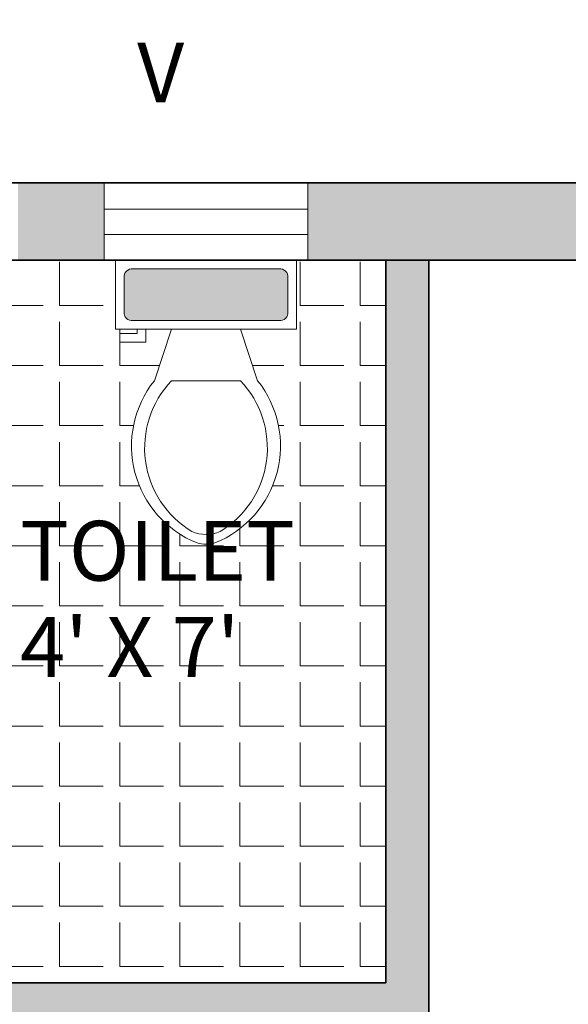
# Model space of a CAD drawing. Units: inches. Extents: x 1858 to 2399, y 1317 to 1943.
# Tile 5 of 8: x 2098 to 2162, y 1742 to 1856. Entities that reach past the tile are written whole.
import ezdxf

# ---------------------------------------------------------------- set-up
doc = ezdxf.new("R2010")
doc.units = ezdxf.units.IN
for name, color, linetype, lineweight in [('A-ANNO-DIMS', 2, 'Continuous', 18), ('A-ANNO-TEXT', 7, 'Continuous', 18), ('A-AREA-IDEN', 7, 'Continuous', 18), ('A-FLOR-FIXT', 9, 'Continuous', 18), ('A-FLOR-FIXT-PATT', 9, 'Continuous', 13), ('A-FLOR-PATT', 8, 'Continuous', 13), ('A-WALL', 7, 'Continuous', 35), ('A-WALL-PATT', 1, 'Continuous', 13), ('window', 4, 'Continuous', 18)]:
    doc.layers.add(name, color=color, linetype=linetype, lineweight=lineweight)
doc.styles.get("Standard").update_dxf_attribs({"font": 'arial.ttf'})
doc.dimstyles.new('ISO-25', dxfattribs={"dimtxt": 12.5, "dimasz": 2.5, "dimexe": 1.25, "dimexo": 0.625, "dimtad": 1, "dimdec": 0, "dimlunit": 4, "dimtxsty": 'Standard', "dimblk": 'ARCHTICK', "dimcen": 2.5, "dimse1": 1, "dimse2": 1, "dimclrd": 3, "dimclrt": 4, "dimadec": 0, "dimazin": 0, "dimtfac": 1, "dimtdec": 0, "dimtmove": 0, "dimatfit": 3, "dimfxl": 1, "dimarcsym": 0})

# ---------------------------------------------------------------- blocks, each defined once
blk = doc.blocks.new('*U4')
for p, q in [((9.5, -6), (9.5, -2)), ((-8, -8.5), (-8, -8)), ((-7, -8), (-7, -9.5)), ((-4, -8), (-6, -14)), ((4, -8), (6, -14)), ((-10, -8.5), (-8, -8.5)), ((-10, -9.5), (-10, -8.5)), ((-7, -9.5), (-10, -9.5)), ((4, -14), (-4, -14))]:
    blk.add_line(p, q)
blk.add_lwpolyline([(10.5, -8), (10.5, 0), (-10.5, 0), (-10.5, -8)], close=True)
for points in [[(8.5, -1), (-8.5, -1)], [(-9.5, -2), (-9.5, -6)], [(-8.5, -7), (8.5, -7)]]:
    blk.add_lwpolyline(points)
for centre, radius, start, end in [((-8.62, -1.88), 0.884, 81.8699, 188.1301), ((8.62, -1.88), 0.884, 351.8699, 98.1301), ((-8.62, -6.12), 0.884, 171.8699, 278.1301), ((8.62, -6.12), 0.884, 261.8699, 8.1301), ((3.52, -21.58), 12.17, 141.4691, 247.9714), ((4.2, -21.82), 11.33, 136.3677, 238.9468), ((-3.52, -21.58), 12.17, 292.0284, 38.5307), ((-4.2, -21.82), 11.33, 301.053, 43.6321), ((0, -27.88), 4, 245.7318, 294.2682), ((0, -29), 4, 254.8605, 285.1395)]:
    blk.add_arc(centre, radius, start, end)
blk = doc.blocks.new('_ArchTick')
at = {"color": 0, "linetype": 'ByBlock', "const_width": 0.15}
blk.add_lwpolyline([(-0.5, -0.5), (0.5, 0.5)], dxfattribs=at)
blk = doc.blocks.new('*D14')
at = {"layer": 'A-ANNO-DIMS', "color": 0, "lineweight": -2, "transparency": 16777216}
blk.add_line((1913.38, 1886.42), (2273.38, 1886.42), dxfattribs=at)
at = {"layer": 'Defpoints', "color": 0, "transparency": 16777216}
for p in [(2273.38, 1886.42), (2273.38, 1827.14), (1913.38, 1826.41)]:
    blk.add_point(p, dxfattribs=at)
at = {"layer": 'A-ANNO-DIMS', "color": 0, "lineweight": -2, "transparency": 16777216, "xscale": 2.5, "yscale": 2.5, "zscale": 2.5, "rotation": 180}
blk.add_blockref('_ArchTick', (1913.38, 1886.42), dxfattribs=at)
at = {"layer": 'A-ANNO-DIMS', "color": 0, "lineweight": -2, "transparency": 16777216, "xscale": 2.5, "yscale": 2.5, "zscale": 2.5}
blk.add_blockref('_ArchTick', (2273.38, 1886.42), dxfattribs=at)
at = {"layer": 'A-ANNO-DIMS', "color": 0, "transparency": 16777216, "insert": (2093.38, 1893.43), "char_height": 12.5, "attachment_point": 5}
blk.add_mtext("30'", dxfattribs=at)
blk = doc.blocks.new('*D33')
at = {"layer": 'A-ANNO-DIMS', "color": 3, "lineweight": -2, "transparency": 16777216}
for p, q in [((1989.86, 1917.54), (2051.43, 1917.54)), ((2051.43, 1917.54), (2117.53, 1917.54))]:
    blk.add_line(p, q, dxfattribs=at)
at = {"layer": 'Defpoints', "color": 0, "transparency": 16777216}
for p in [(2051.43, 1917.54), (1989.86, 1837.34), (2051.43, 1837.34)]:
    blk.add_point(p, dxfattribs=at)
at = {"layer": 'A-ANNO-DIMS', "color": 3, "lineweight": -2, "transparency": 16777216, "xscale": 2.5, "yscale": 2.5, "zscale": 2.5, "rotation": 180}
blk.add_blockref('_ArchTick', (1989.86, 1917.54), dxfattribs=at)
at = {"layer": 'A-ANNO-DIMS', "color": 3, "lineweight": -2, "transparency": 16777216, "xscale": 2.5, "yscale": 2.5, "zscale": 2.5}
blk.add_blockref('_ArchTick', (2051.43, 1917.54), dxfattribs=at)
at = {"layer": 'A-ANNO-DIMS', "color": 4, "transparency": 16777216, "insert": (2085.73, 1924.63), "char_height": 12.5, "attachment_point": 5}
blk.add_mtext('5\'-1 1/2"', dxfattribs=at)
blk = doc.blocks.new('*D34')
at = {"layer": 'A-ANNO-DIMS', "color": 3, "lineweight": -2, "transparency": 16777216}
blk.add_line((2051.43, 1917.54), (2107.67, 1917.54), dxfattribs=at)
at = {"layer": 'Defpoints', "color": 0, "transparency": 16777216}
for p in [(2107.67, 1917.54), (2051.43, 1837.34), (2107.67, 1837.34)]:
    blk.add_point(p, dxfattribs=at)
at = {"layer": 'A-ANNO-DIMS', "color": 3, "lineweight": -2, "transparency": 16777216, "xscale": 2.5, "yscale": 2.5, "zscale": 2.5, "rotation": 180}
blk.add_blockref('_ArchTick', (2051.43, 1917.54), dxfattribs=at)
at = {"layer": 'A-ANNO-DIMS', "color": 3, "lineweight": -2, "transparency": 16777216, "xscale": 2.5, "yscale": 2.5, "zscale": 2.5}
blk.add_blockref('_ArchTick', (2107.67, 1917.54), dxfattribs=at)
at = {"layer": 'A-ANNO-DIMS', "color": 4, "transparency": 16777216, "insert": (2079.55, 1924.55), "char_height": 12.5, "attachment_point": 5}
blk.add_mtext('4\'-8"', dxfattribs=at)
blk = doc.blocks.new('*D35')
at = {"layer": 'A-ANNO-DIMS', "color": 3, "lineweight": -2, "transparency": 16777216}
for p, q in [((2107.67, 1917.54), (2131.33, 1917.54)), ((2131.33, 1917.54), (2205.97, 1917.54))]:
    blk.add_line(p, q, dxfattribs=at)
at = {"layer": 'Defpoints', "color": 0, "transparency": 16777216}
for p in [(2131.33, 1917.54), (2107.67, 1837.34), (2131.33, 1837.34)]:
    blk.add_point(p, dxfattribs=at)
at = {"layer": 'A-ANNO-DIMS', "color": 3, "lineweight": -2, "transparency": 16777216, "xscale": 2.5, "yscale": 2.5, "zscale": 2.5, "rotation": 180}
blk.add_blockref('_ArchTick', (2107.67, 1917.54), dxfattribs=at)
at = {"layer": 'A-ANNO-DIMS', "color": 3, "lineweight": -2, "transparency": 16777216, "xscale": 2.5, "yscale": 2.5, "zscale": 2.5}
blk.add_blockref('_ArchTick', (2131.33, 1917.54), dxfattribs=at)
at = {"layer": 'A-ANNO-DIMS', "color": 4, "transparency": 16777216, "insert": (2169.9, 1924.63), "char_height": 12.5, "attachment_point": 5}
blk.add_mtext('1\'-11 1/2"', dxfattribs=at)
blk = doc.blocks.new('*D36')
at = {"layer": 'A-ANNO-DIMS', "color": 3, "lineweight": -2, "transparency": 16777216}
for p, q in [((2131.33, 1917.54), (2186.7, 1917.54)), ((2186.7, 1917.54), (2253.31, 1917.54))]:
    blk.add_line(p, q, dxfattribs=at)
at = {"layer": 'Defpoints', "color": 0, "transparency": 16777216}
for p in [(2186.7, 1917.54), (2131.33, 1837.34), (2186.7, 1837.34)]:
    blk.add_point(p, dxfattribs=at)
at = {"layer": 'A-ANNO-DIMS', "color": 3, "lineweight": -2, "transparency": 16777216, "xscale": 2.5, "yscale": 2.5, "zscale": 2.5, "rotation": 180}
blk.add_blockref('_ArchTick', (2131.33, 1917.54), dxfattribs=at)
at = {"layer": 'A-ANNO-DIMS', "color": 3, "lineweight": -2, "transparency": 16777216, "xscale": 2.5, "yscale": 2.5, "zscale": 2.5}
blk.add_blockref('_ArchTick', (2186.7, 1917.54), dxfattribs=at)
at = {"layer": 'A-ANNO-DIMS', "color": 4, "transparency": 16777216, "insert": (2221.25, 1924.63), "char_height": 12.5, "attachment_point": 5}
blk.add_mtext('4\'-7 1/2"', dxfattribs=at)
blk = doc.blocks.new('*D50')
at = {"layer": 'A-ANNO-DIMS', "color": 3, "lineweight": -2, "transparency": 16777216}
for p, q in [((2097.46, 1917.54), (2127.41, 1917.54)), ((2127.41, 1917.54), (2164.6, 1917.54))]:
    blk.add_line(p, q, dxfattribs=at)
at = {"layer": 'Defpoints', "color": 0, "transparency": 16777216}
for p in [(2127.41, 1917.54), (2097.46, 1563.34), (2127.41, 1563.34)]:
    blk.add_point(p, dxfattribs=at)
at = {"layer": 'A-ANNO-DIMS', "color": 3, "lineweight": -2, "transparency": 16777216, "xscale": 2.5, "yscale": 2.5, "zscale": 2.5, "rotation": 180}
blk.add_blockref('_ArchTick', (2097.46, 1917.54), dxfattribs=at)
at = {"layer": 'A-ANNO-DIMS', "color": 3, "lineweight": -2, "transparency": 16777216, "xscale": 2.5, "yscale": 2.5, "zscale": 2.5}
blk.add_blockref('_ArchTick', (2127.41, 1917.54), dxfattribs=at)
at = {"layer": 'A-ANNO-DIMS', "color": 4, "transparency": 16777216, "insert": (2147.25, 1924.55), "char_height": 12.5, "attachment_point": 5}
blk.add_mtext('2\'-6"', dxfattribs=at)
blk = doc.blocks.new('*D51')
at = {"layer": 'A-ANNO-DIMS', "color": 3, "lineweight": -2, "transparency": 16777216}
for p, q in [((2127.41, 1917.54), (2171.86, 1917.54)), ((2171.86, 1917.54), (2237.95, 1917.54))]:
    blk.add_line(p, q, dxfattribs=at)
at = {"layer": 'Defpoints', "color": 0, "transparency": 16777216}
for p in [(2171.86, 1917.54), (2127.41, 1563.34), (2171.86, 1563.34)]:
    blk.add_point(p, dxfattribs=at)
at = {"layer": 'A-ANNO-DIMS', "color": 3, "lineweight": -2, "transparency": 16777216, "xscale": 2.5, "yscale": 2.5, "zscale": 2.5, "rotation": 180}
blk.add_blockref('_ArchTick', (2127.41, 1917.54), dxfattribs=at)
at = {"layer": 'A-ANNO-DIMS', "color": 3, "lineweight": -2, "transparency": 16777216, "xscale": 2.5, "yscale": 2.5, "zscale": 2.5}
blk.add_blockref('_ArchTick', (2171.86, 1917.54), dxfattribs=at)
at = {"layer": 'A-ANNO-DIMS', "color": 4, "transparency": 16777216, "insert": (2206.15, 1924.63), "char_height": 12.5, "attachment_point": 5}
blk.add_mtext('3\'-8 1/2"', dxfattribs=at)
blk = doc.blocks.new('*D58')
at = {"layer": 'A-ANNO-DIMS', "color": 3, "lineweight": -2, "transparency": 16777216}
for p, q in [((1884.18, 1730.57), (1884.18, 1767.76)), ((1884.18, 1706.78), (1884.18, 1730.57))]:
    blk.add_line(p, q, dxfattribs=at)
at = {"layer": 'Defpoints', "color": 0, "transparency": 16777216}
for p in [(1884.18, 1730.57), (2145.38, 1730.57), (2145.38, 1706.78)]:
    blk.add_point(p, dxfattribs=at)
at = {"layer": 'A-ANNO-DIMS', "color": 3, "lineweight": -2, "transparency": 16777216, "xscale": 2.5, "yscale": 2.5, "zscale": 2.5}
for p, rotation in [((1884.18, 1730.57), 90), ((1884.18, 1706.78), 270)]:
    blk.add_blockref('_ArchTick', p, dxfattribs=dict(at, rotation=rotation))
at = {"layer": 'A-ANNO-DIMS', "color": 4, "transparency": 16777216, "insert": (1877.17, 1750.41), "char_height": 12.5, "attachment_point": 5, "rotation": 90}
blk.add_mtext('2\'-0"', dxfattribs=at)

msp = doc.modelspace()

# ---------------------------------------------------------------- hatches: boundary and pattern name
at = {"layer": 'A-FLOR-FIXT-PATT'}
h = msp.add_hatch(color=256, dxfattribs=at)
h.dxf.hatch_style = 1
h.set_gradient(color1=(0, 0, 255), color2=(255, 255, 0))
h.paths.add_polyline_path([(2010.03, 1501.34), (2040.03, 1501.34), (2040.03, 1477.34), (2034.03, 1477.34), (2034.03, 1476.34), (2038.03, 1476.34), (2050.44, 1476.34), (2056.5, 1476.34), (2056.5, 1507.28), (1988.35, 1507.28), (1988.35, 1554.34), (1967.38, 1554.34), (1967.38, 1525.7, -0.414214), (1968.88, 1527.2), (1985.88, 1527.2, -0.414214), (1987.38, 1525.7), (1987.38, 1498.7, -0.414214), (1985.88, 1497.2), (1968.88, 1497.2, -0.414214), (1967.38, 1498.7), (1967.38, 1476.34), (2016.03, 1476.34), (2016.03, 1477.34), (2010.03, 1477.34)])
h.paths.add_polyline_path([(2129, 1826.59, 0.414214), (2128, 1827.34), (2110.75, 1827.34, 0.414214), (2110, 1826.34), (2110, 1822.09, 0.414214), (2111, 1821.34), (2128.25, 1821.34, 0.414214), (2129, 1822.34)])
h.paths.add_polyline_path([(2047.65, 1651.34), (2026.65, 1651.34), (2026.65, 1643.34), (2047.65, 1643.34)])
h.paths.add_polyline_path([(2045.65, 1644.34, 0.5), (2046.65, 1645.34), (2046.65, 1649.34, 0.5), (2045.65, 1650.34), (2028.65, 1650.34, 0.5), (2027.65, 1649.34), (2027.65, 1645.34, 0.5), (2028.65, 1644.34)], flags=16)
at = {"layer": 'A-FLOR-PATT'}
h = msp.add_hatch(dxfattribs=at)
h.set_pattern_fill('ANGLE', color=256)
h.set_pattern_definition([(0, (0, 0), (0, 6.985), [5.08, -1.905]), (90, (0, 0), (-6.985, 4e-16), [5.08, -1.905])])
h.paths.add_polyline_path([(2058.38, 1691.34), (2005.38, 1691.34), (2005.38, 1696.34), (1977.99, 1696.34), (1977.99, 1691.34), (1967.38, 1691.34), (1967.38, 1643.34), (2026.65, 1643.34), (2026.65, 1651.34), (2033.15, 1651.34), (2031.15, 1657.34, -0.501323), (2036.1, 1676.2, -0.132891), (2038.19, 1676.2, -0.501317), (2043.15, 1657.34), (2041.15, 1651.34), (2044.15, 1651.34), (2044.15, 1652.84), (2047.15, 1652.84), (2047.15, 1651.34), (2047.65, 1651.34), (2047.65, 1643.34), (2058.38, 1643.34)])
h.paths.add_polyline_path([(2140.38, 1828.34), (2130, 1828.34), (2130, 1820.34), (2123.5, 1820.34), (2125.5, 1814.34, -0.501323), (2120.55, 1795.48, -0.132891), (2118.46, 1795.48, -0.501317), (2113.5, 1814.34), (2115.5, 1820.34), (2112.5, 1820.34), (2112.5, 1818.84), (2109.5, 1818.84), (2109.5, 1820.34), (2109, 1820.34), (2109, 1828.34), (2107.67, 1828.34), (2092.38, 1828.34), (2092.38, 1744.34), (2140.38, 1744.34)])
h.paths.add_polyline_path([(1981.03, 1683.02), (1996.96, 1683.02), (1996.96, 1693.5), (1981.03, 1693.5)], flags=24)
h.paths.add_polyline_path([(1975.79, 1660.59), (2014.55, 1660.59), (2014.55, 1671.04), (1975.79, 1671.04)], flags=24)
h.paths.add_polyline_path([(1975.73, 1671.6), (2013.37, 1671.6), (2013.37, 1682.41), (1975.73, 1682.41)], flags=24)
h.paths.add_polyline_path([(2096.15, 1778.17), (2126.05, 1778.17), (2126.05, 1788.61), (2096.15, 1788.61)], flags=24)
h.paths.add_polyline_path([(2096.09, 1789.17), (2133.73, 1789.17), (2133.73, 1799.98), (2096.09, 1799.98)], flags=24)
at = {"layer": 'A-WALL-PATT'}
h = msp.add_hatch(color=256, dxfattribs=at)
h.dxf.hatch_style = 1
h.paths.add_polyline_path([(1967.38, 1742.58), (1958.38, 1742.58), (1958.38, 1700.89), (1967.38, 1700.89)])
h.paths.add_polyline_path([(1967.38, 1685.05), (1958.38, 1685.05), (1958.38, 1672.42), (1967.38, 1672.42)], flags=17)
h.paths.add_polyline_path([(2092.38, 1643.34), (2087.38, 1643.34), (2063.38, 1643.34), (2063.38, 1691.34), (2087.38, 1691.34), (2092.38, 1691.34), (2092.38, 1696.34), (2087.38, 1696.34), (2005.38, 1696.34), (2005.38, 1691.34), (2058.38, 1691.34), (2058.38, 1643.34), (1967.38, 1643.34), (1967.38, 1652.51), (1958.38, 1652.51), (1958.38, 1625.4), (1967.38, 1625.4), (1967.38, 1638.34), (2087.38, 1638.34), (2087.38, 1617.63), (2092.38, 1617.63)])
h.paths.add_polyline_path([(1967.38, 1591.74), (1958.38, 1591.74), (1958.38, 1571.83), (1967.38, 1571.83)])
h.paths.add_polyline_path([(1967.38, 1554.34), (2002.1, 1554.34), (2002.1, 1559.34), (1967.38, 1559.34), (1958.38, 1559.34), (1958.38, 1536.07), (1967.38, 1536.07)])
h.paths.add_polyline_path([(2087.38, 1559.34), (2042.3, 1559.34), (2042.3, 1554.34), (2087.38, 1554.34)])
h.paths.add_polyline_path([(2092.38, 1583.24), (2087.38, 1583.24), (2087.38, 1563.34), (2092.38, 1563.34)])
h.paths.add_polyline_path([(2096.38, 1554.34), (2087.38, 1554.34), (2087.38, 1481.51), (2096.38, 1473.96)])
h.paths.add_polyline_path([(2084.48, 1476.34), (2050.44, 1476.34), (2050.44, 1467.34), (2089.85, 1467.34)])
h.paths.add_polyline_path([(2002.33, 1476.34), (1977.97, 1476.34), (1967.38, 1467.34), (2002.33, 1467.34)])
h.paths.add_polyline_path([(1967.38, 1488.33), (1958.38, 1488.33), (1958.38, 1474.25), (1967.38, 1482.01)])
h.paths.add_polyline_path([(2121.99, 1554.34), (2119.71, 1554.34), (2119.71, 1532.61), (2096.38, 1532.61), (2096.38, 1529.65), (2121.99, 1529.65)])
h.paths.add_polyline_path([(2171.86, 1563.34), (2127.41, 1563.34), (2127.41, 1554.34), (2171.86, 1554.34)])
h.paths.add_polyline_path([(2264.38, 1563.34), (2220, 1563.34), (2220, 1554.34), (2264.38, 1554.34)])
h.paths.add_polyline_path([(2273.38, 1563.34), (2264.38, 1563.34), (2264.38, 1366.34), (2241.64, 1366.34), (2241.64, 1357.34), (2273.38, 1357.34)])
h.paths.add_polyline_path([(2273.38, 1691.34), (2264.38, 1691.34), (2264.38, 1576.35), (2273.38, 1576.35)])
h.paths.add_polyline_path([(2273.38, 1827.14), (2264.38, 1823.36), (2264.38, 1706.46), (2273.38, 1706.46)])
h.paths.add_polyline_path([(2265.79, 1837.34), (2234.56, 1837.34), (2234.56, 1828.34), (2258.24, 1828.34)])
h.paths.add_polyline_path([(2186.7, 1837.34), (2131.33, 1837.34), (2131.33, 1828.34), (2186.7, 1828.34)])
h.paths.add_polyline_path([(2107.67, 1837.34), (2097.64, 1837.34), (2097.64, 1828.34), (2107.67, 1828.34)])
h.paths.add_polyline_path([(2082.58, 1837.34), (2051.43, 1837.34), (2051.43, 1828.34), (2082.58, 1828.34)])
h.paths.add_polyline_path([(2092.38, 1828.34), (2087.38, 1828.34), (2087.38, 1729.93), (2092.38, 1729.93), (2092.38, 1739.34), (2140.38, 1739.34), (2140.38, 1730.57), (2145.38, 1730.57), (2145.38, 1828.34), (2140.38, 1828.34), (2140.38, 1744.34), (2092.38, 1744.34)])
h.paths.add_polyline_path([(1989.86, 1837.34), (1977.66, 1837.34), (1977.66, 1828.34), (1989.86, 1828.34)])
h.paths.add_polyline_path([(1922.38, 1822.27), (1913.38, 1826.41), (1913.38, 1357.34), (1951.36, 1357.34), (1951.36, 1366.34), (1922.38, 1366.34)])
h.paths.add_polyline_path([(1967.38, 1828.34), (1958.38, 1828.34), (1958.38, 1791.57), (1967.38, 1791.57)])

# ---------------------------------------------------------------- linework, layer by layer
at = {"layer": 'A-WALL'}
for p, q in [((1949.42, 1828.34), (2264.38, 1828.34)), ((2140.38, 1744.34), (2140.38, 1828.34)), ((2145.38, 1730.57), (2145.38, 1828.34)), ((2092.38, 1744.34), (2140.38, 1744.34))]:
    msp.add_line(p, q, dxfattribs=at)
msp.add_lwpolyline([(1949.42, 1837.34), (2273.38, 1837.34), (2273.38, 1357.34), (1913.38, 1357.34), (1913.38, 1826.41)], dxfattribs=at)
at = {"layer": 'window'}
for p, q in [((2107.67, 1837.34), (2107.67, 1828.34)), ((2131.33, 1837.34), (2107.67, 1837.34)), ((2131.33, 1828.34), (2131.33, 1837.34)), ((2131.33, 1834.28), (2107.67, 1834.28)), ((2131.33, 1831.34), (2107.67, 1831.34)), ((2107.67, 1828.34), (2131.33, 1828.34))]:
    msp.add_line(p, q, dxfattribs=at)

# ---------------------------------------------------------------- block references
at = {"layer": 'A-FLOR-FIXT'}
msp.add_blockref('*U4', (2119.5, 1828.34), dxfattribs=at)

# ---------------------------------------------------------------- texts
at = {"layer": 'A-ANNO-TEXT'}
msp.add_text('V', height=6.96, dxfattribs=at).set_placement((2111.5, 1846.69))
at = {"layer": 'A-AREA-IDEN'}
for s, p in [('TOILET', (2097.89, 1791.09)), ("4' X 7'", (2097.89, 1779.91))]:
    msp.add_text(s, height=6.96, dxfattribs=at).set_placement(p)

# ---------------------------------------------------------------- dimensions: what is measured, and where the dimension line sits
at = {"layer": 'A-ANNO-DIMS'}
for base, p1, p2, override, picture, middle in [((2051.43, 1917.54), (1989.86, 1837.34), (2051.43, 1837.34), {"dimdec": 1, "dimlfac": 1, "dimrnd": 0, "dimzin": 1, "dimdsep": 46, "dimlunit": 4, "dimfrac": 2}, '*D33', (2085.73, 1924.63)), ((2131.33, 1917.54), (2107.67, 1837.34), (2131.33, 1837.34), {"dimdec": 1, "dimlfac": 1, "dimrnd": 0, "dimzin": 1, "dimdsep": 46, "dimlunit": 4, "dimfrac": 2}, '*D35', (2169.9, 1924.63)), ((2171.8564, 1917.5395), (2127.4089, 1563.3395), (2171.8564, 1563.3395), {"dimdec": 1, "dimlfac": 1, "dimrnd": 0, "dimzin": 1, "dimdsep": 46, "dimlunit": 4, "dimfrac": 2}, '*D51', (2206.1547, 1924.6319)), ((2186.7, 1917.54), (2131.33, 1837.34), (2186.7, 1837.34), {"dimdec": 1, "dimlfac": 1, "dimrnd": 0, "dimzin": 1, "dimdsep": 46, "dimlunit": 4, "dimfrac": 2}, '*D36', (2221.25, 1924.63)), ((2107.67, 1917.54), (2051.43, 1837.34), (2107.67, 1837.34), {"dimdec": 1, "dimlfac": 1, "dimrnd": 0, "dimzin": 1, "dimdsep": 46, "dimlunit": 4, "dimfrac": 2}, '*D34', (2079.55, 1924.55)), ((2127.4089, 1917.5395), (2097.4626, 1563.3395), (2127.4089, 1563.3395), {"dimdec": 1, "dimlfac": 1, "dimrnd": 0, "dimzin": 1, "dimdsep": 46, "dimlunit": 4, "dimfrac": 2}, '*D50', (2147.2545, 1924.5467)), ((2273.38, 1886.42), (1913.38, 1826.41), (2273.38, 1827.14), {"dimclrd": 0, "dimclre": 0, "dimclrt": 0}, '*D14', (2093.38, 1893.43))]:
    dim = msp.add_linear_dim(base=base, p1=p1, p2=p2, dimstyle='ISO-25', override=override, dxfattribs=at)
    dim.commit()
    dim.dimension.update_dxf_attribs({"geometry": picture, "text_midpoint": middle})
dim = msp.add_linear_dim(base=(1884.18, 1730.57), p1=(2145.38, 1706.78), p2=(2145.38, 1730.57), angle=90, dimstyle='ISO-25', override={"dimdec": 1, "dimlfac": 1, "dimrnd": 0, "dimzin": 1, "dimdsep": 46, "dimlunit": 4, "dimfrac": 2}, dxfattribs=at)
dim.commit()
dim.dimension.update_dxf_attribs({"geometry": '*D58', "text_midpoint": (1877.17, 1750.41)})

doc.saveas('drawing.dxf')
